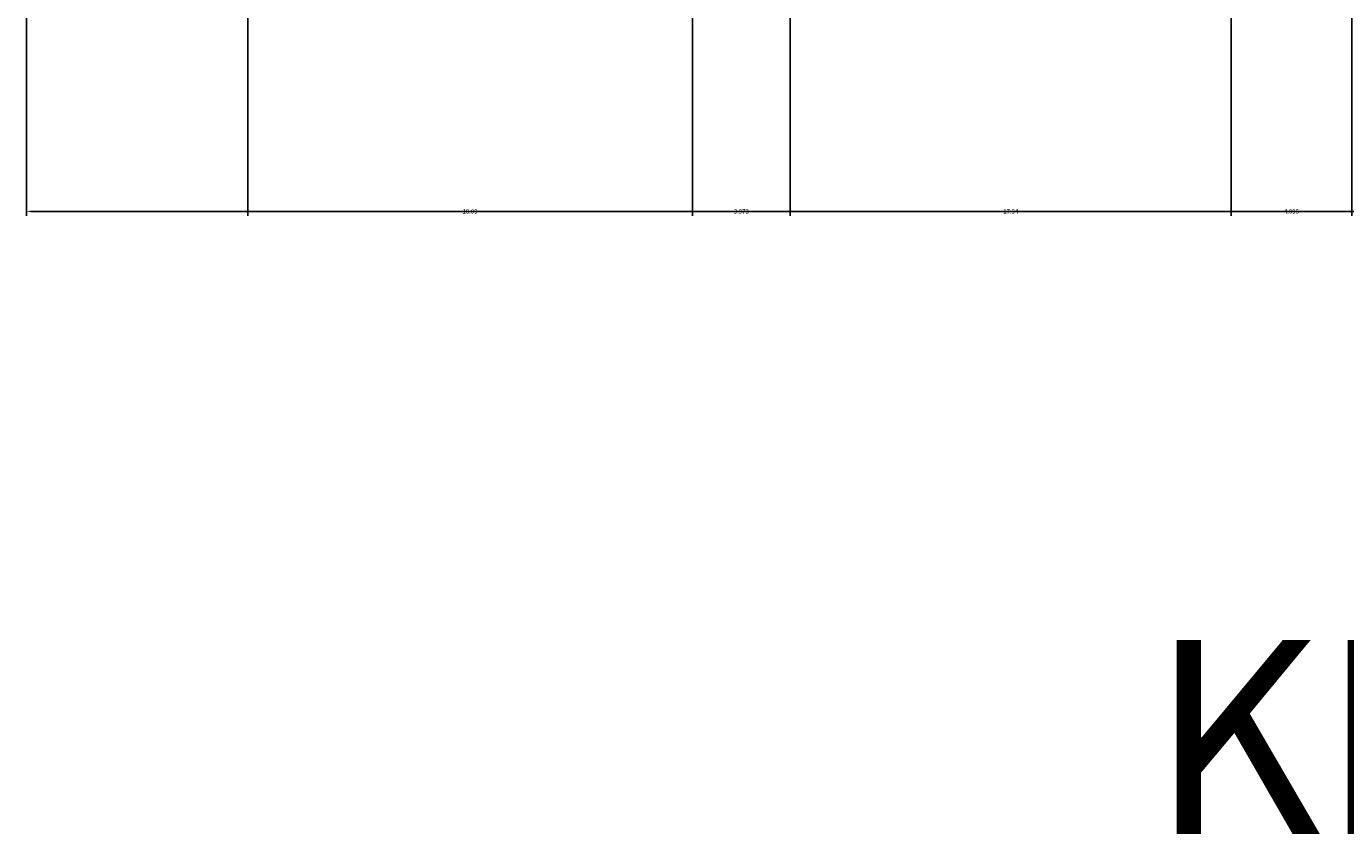
# Model space of a CAD drawing. Units: inches. Extents: x 27 to 200, y -50 to 102.
# Tile 1 of 26: x 35 to 89, y -50 to -17. Entities that reach past the tile are written whole.
import ezdxf

# ---------------------------------------------------------------- set-up
doc = ezdxf.new("R2010")
doc.units = ezdxf.units.IN
doc.header["$MEASUREMENT"] = 0
doc.layers.add('A-ANNO-DIMS', color=2, linetype='Continuous', lineweight=18)
doc.layers.add('A-ANNO-TEXT', color=3, linetype='Continuous', lineweight=25)
doc.styles.get("Standard").update_dxf_attribs({"font": 'arial.ttf'})
doc.dimstyles.get("Standard").update_dxf_attribs({"dimtxt": 0.18, "dimasz": 0.18, "dimexe": 0.18, "dimexo": 0.0625, "dimgap": 0.09, "dimtad": 0, "dimtih": 1, "dimtoh": 1, "dimdec": 4, "dimzin": 0, "dimdsep": 46, "dimtxsty": 'Standard', "dimcen": 0.09, "dimadec": 0, "dimazin": 0, "dimtfac": 1, "dimtdec": 4, "dimtofl": 0, "dimtmove": 0, "dimatfit": 3, "dimfxl": 1, "dimtolj": 1, "dimtzin": 0, "dimarcsym": 0})

# ---------------------------------------------------------------- blocks, each defined once
blk = doc.blocks.new('*D23')
at = {"layer": 'A-ANNO-DIMS', "color": 0, "lineweight": -2, "transparency": 16777216}
for p, q in [((35.417, -16.832), (35.417, -25.149)), ((191.417, -16.832), (191.417, -25.149)), ((35.597, -24.969), (113.137, -24.969)), ((191.237, -24.969), (113.697, -24.969))]:
    blk.add_line(p, q, dxfattribs=at)
at = {"layer": 'A-ANNO-DIMS', "color": 0, "transparency": 16777216}
for points in [[(35.597, -24.939), (35.597, -24.999), (35.417, -24.969)], [(191.237, -24.939), (191.237, -24.999), (191.417, -24.969)]]:
    blk.add_solid(points, dxfattribs=at)
at = {"layer": 'Defpoints', "color": 0, "transparency": 16777216}
for p in [(35.417, -16.769), (191.417, -16.769), (191.417, -24.969)]:
    blk.add_point(p, dxfattribs=at)
at = {"layer": 'A-ANNO-DIMS', "color": 0, "transparency": 16777216, "insert": (113.417, -24.969), "char_height": 0.18, "attachment_point": 5}
blk.add_mtext('\\A1;156', dxfattribs=at)
blk = doc.blocks.new('*D33')
at = {"layer": 'A-ANNO-DIMS', "color": 0, "lineweight": -2, "transparency": 16777216}
for p, q in [((84.417, -16.832), (84.417, -25.149)), ((89.312, -16.832), (89.312, -25.149)), ((84.597, -24.969), (86.466, -24.969)), ((89.132, -24.969), (87.262, -24.969))]:
    blk.add_line(p, q, dxfattribs=at)
at = {"layer": 'A-ANNO-DIMS', "color": 0, "transparency": 16777216}
for points in [[(84.597, -24.939), (84.597, -24.999), (84.417, -24.969)], [(89.132, -24.939), (89.132, -24.999), (89.312, -24.969)]]:
    blk.add_solid(points, dxfattribs=at)
at = {"layer": 'Defpoints', "color": 0, "transparency": 16777216}
for p in [(84.417, -16.769), (89.312, -16.769), (89.312, -24.969)]:
    blk.add_point(p, dxfattribs=at)
at = {"layer": 'A-ANNO-DIMS', "color": 0, "transparency": 16777216, "insert": (86.864, -24.969), "char_height": 0.18, "attachment_point": 5}
blk.add_mtext('\\A1;4.895', dxfattribs=at)
blk = doc.blocks.new('*D41')
at = {"layer": 'A-ANNO-DIMS', "color": 0, "lineweight": -2, "transparency": 16777216}
for p, q in [((62.505, -3.679), (62.505, -25.149)), ((44.417, -16.832), (44.417, -25.149)), ((44.597, -24.969), (53.076, -24.969)), ((62.325, -24.969), (53.847, -24.969))]:
    blk.add_line(p, q, dxfattribs=at)
at = {"layer": 'A-ANNO-DIMS', "color": 0, "transparency": 16777216}
for points in [[(44.597, -24.939), (44.597, -24.999), (44.417, -24.969)], [(62.325, -24.939), (62.325, -24.999), (62.505, -24.969)]]:
    blk.add_solid(points, dxfattribs=at)
at = {"layer": 'Defpoints', "color": 0, "transparency": 16777216}
for p in [(62.505, -3.617), (44.417, -16.769), (62.505, -24.969)]:
    blk.add_point(p, dxfattribs=at)
at = {"layer": 'A-ANNO-DIMS', "color": 0, "transparency": 16777216, "insert": (53.461, -24.969), "char_height": 0.18, "attachment_point": 5}
blk.add_mtext('\\A1;18.09', dxfattribs=at)
blk = doc.blocks.new('*D42')
at = {"layer": 'A-ANNO-DIMS', "color": 0, "lineweight": -2, "transparency": 16777216}
for p, q in [((62.505, -3.679), (62.505, -25.149)), ((66.479, -3.679), (66.479, -25.149)), ((62.685, -24.969), (64.098, -24.969)), ((66.299, -24.969), (64.886, -24.969))]:
    blk.add_line(p, q, dxfattribs=at)
at = {"layer": 'A-ANNO-DIMS', "color": 0, "transparency": 16777216}
for points in [[(62.685, -24.939), (62.685, -24.999), (62.505, -24.969)], [(66.299, -24.939), (66.299, -24.999), (66.479, -24.969)]]:
    blk.add_solid(points, dxfattribs=at)
at = {"layer": 'Defpoints', "color": 0, "transparency": 16777216}
for p in [(62.505, -3.617), (66.479, -3.617), (66.479, -24.969)]:
    blk.add_point(p, dxfattribs=at)
at = {"layer": 'A-ANNO-DIMS', "color": 0, "transparency": 16777216, "insert": (64.492, -24.969), "char_height": 0.18, "attachment_point": 5}
blk.add_mtext('\\A1;3.973', dxfattribs=at)
blk = doc.blocks.new('*D43')
at = {"layer": 'A-ANNO-DIMS', "color": 0, "lineweight": -2, "transparency": 16777216}
for p, q in [((66.479, -3.679), (66.479, -25.149)), ((84.417, -16.832), (84.417, -25.149)), ((66.659, -24.969), (75.063, -24.969)), ((84.237, -24.969), (75.833, -24.969))]:
    blk.add_line(p, q, dxfattribs=at)
at = {"layer": 'A-ANNO-DIMS', "color": 0, "transparency": 16777216}
for points in [[(66.659, -24.939), (66.659, -24.999), (66.479, -24.969)], [(84.237, -24.939), (84.237, -24.999), (84.417, -24.969)]]:
    blk.add_solid(points, dxfattribs=at)
at = {"layer": 'Defpoints', "color": 0, "transparency": 16777216}
for p in [(66.479, -3.617), (84.417, -16.769), (84.417, -24.969)]:
    blk.add_point(p, dxfattribs=at)
at = {"layer": 'A-ANNO-DIMS', "color": 0, "transparency": 16777216, "insert": (75.448, -24.969), "char_height": 0.18, "attachment_point": 5}
blk.add_mtext('\\A1;17.94', dxfattribs=at)

msp = doc.modelspace()

# ---------------------------------------------------------------- texts
at = {"layer": 'A-ANNO-TEXT'}
msp.add_text('KITCHEN ELEVATION ', height=7.893413, dxfattribs=at).set_placement((81.1084, -50.2843))

# ---------------------------------------------------------------- dimensions: what is measured, and where the dimension line sits
at = {"layer": 'A-ANNO-DIMS'}
for base, p1, p2, override, picture, middle in [((62.5054, -24.9693), (44.4169, -16.7693), (62.5054, -3.6168), {"dimdec": 2, "dimlfac": 1, "dimrnd": 0, "dimzin": 0, "dimdsep": 46, "dimlunit": 2}, '*D41', (53.4611, -24.9693)), ((66.4786, -24.9693), (62.5054, -3.6168), (66.4786, -3.6168), {"dimdec": 3, "dimlfac": 1, "dimrnd": 0, "dimzin": 0, "dimdsep": 46, "dimlunit": 2}, '*D42', (64.492, -24.9693)), ((84.4169, -24.9693), (66.4786, -3.6168), (84.4169, -16.7693), {"dimdec": 2, "dimlfac": 1, "dimrnd": 0, "dimzin": 0, "dimdsep": 46, "dimlunit": 2}, '*D43', (75.4478, -24.9693)), ((191.4169, -24.9693), (35.4169, -16.7693), (191.4169, -16.7693), {"dimdec": 0, "dimlfac": 1, "dimrnd": 0, "dimzin": 0, "dimdsep": 46, "dimlunit": 2}, '*D23', (113.4169, -24.9693)), ((89.3118, -24.9693), (84.4169, -16.7693), (89.3118, -16.7693), {"dimdec": 3, "dimlfac": 1, "dimrnd": 0, "dimzin": 0, "dimdsep": 46, "dimlunit": 2}, '*D33', (86.8644, -24.9693))]:
    dim = msp.add_linear_dim(base=base, p1=p1, p2=p2, dimstyle='Standard', override=override, dxfattribs=at)
    dim.commit()
    dim.dimension.update_dxf_attribs({"geometry": picture, "text_midpoint": middle})

doc.saveas('drawing.dxf')
